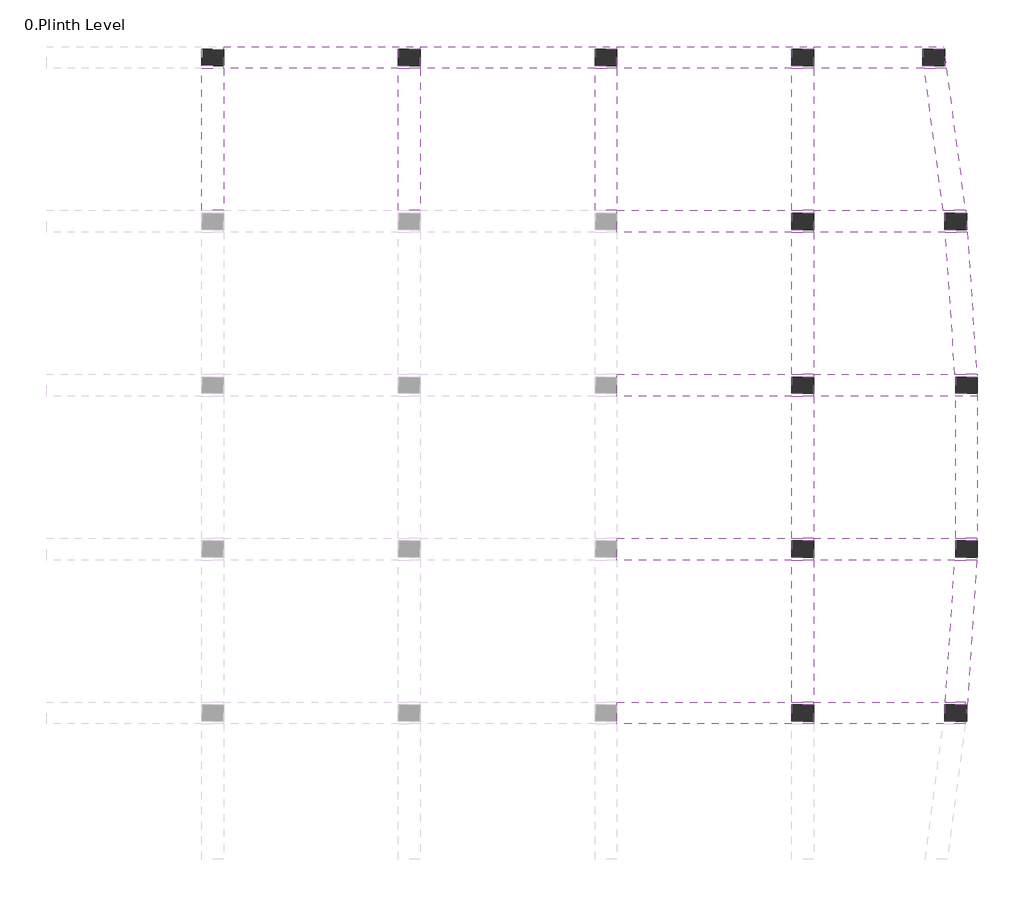
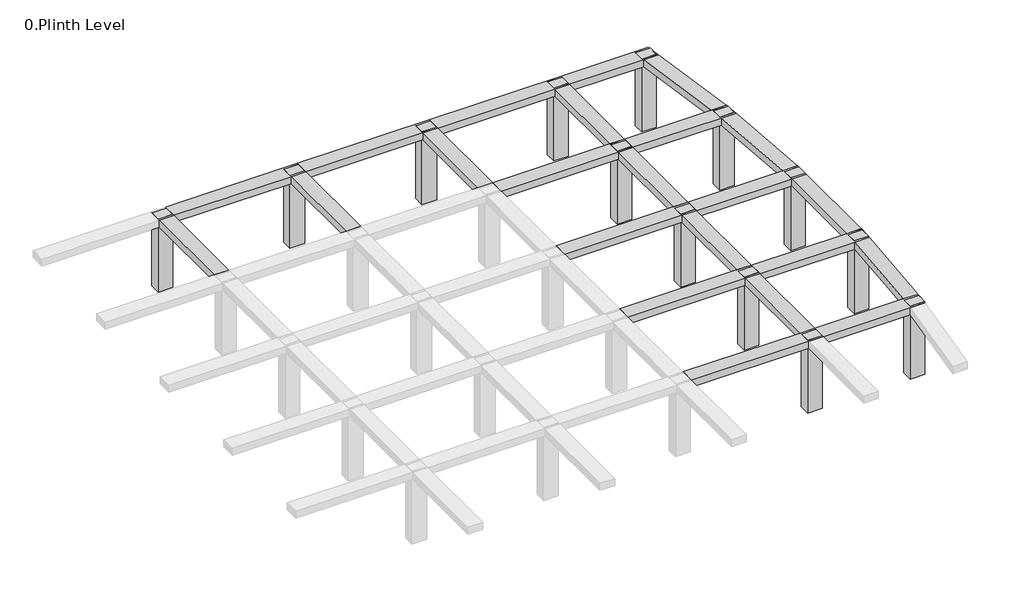
# One storey, part 3 of 3: 23 beams, 13 columns.
"""IFC4 building model written with IfcOpenShell, lengths in millimetres."""

from ifc_helpers import new_model, si_unit, frame, origin, origin_with_axes, place, context, project, spatial, polyline, outline, extrude, faceted_brep, element, save

model = new_model("IFC4")

# Units and contexts
model_context = context("Model", 3, world=origin())
ifc_project = project(units=[si_unit("LENGTHUNIT", "METRE", prefix="MILLI")], contexts=[model_context])

# Site, building, storey
site = spatial("IfcSite", under=ifc_project)
building = spatial("IfcBuilding", under=site)
storey = spatial("IfcBuildingStorey", under=building, Name="0.Plinth Level", Elevation=0.0)

# Beams
placement = place(None, origin())
element("IfcBeam", 1, ObjectType="Concrete-Rectangular Beam : 2' x2'", at=placement, inside=storey, context=model_context, shape_type="Brep", body=[
    faceted_brep([(-160.074232, 1680.7831222, 3200.4), (-160.074232, 1604.5831222, 3200.4), (-160.074232, 1147.3831222, 3200.4), (-160.074232, 1071.1831222, 3200.4), (4716.725768, 1071.1831222, 3200.4), (5326.325768, 1071.1831222, 3200.4), (5326.325768, 1147.3831222, 3200.4), (4716.725768, 1147.3831222, 3200.4), (4716.725768, 1604.5831222, 3200.4), (5326.325768, 1604.5831222, 3200.4), (5326.325768, 1680.7831222, 3200.4), (4716.725768, 1680.7831222, 3200.4), (-160.074232, 1071.1831222, 2895.6), (4716.725768, 1071.1831222, 2895.6), (5326.325768, 1071.1831222, 2895.6), (-160.074232, 1147.3831222, 2895.6), (-160.074232, 1604.5831222, 2895.6), (-160.074232, 1680.7831222, 2895.6), (4716.725768, 1680.7831222, 2895.6), (5326.325768, 1680.7831222, 2895.6), (5326.325768, 1604.5831222, 2895.6), (4716.725768, 1604.5831222, 2895.6), (4716.725768, 1147.3831222, 2895.6), (5326.325768, 1147.3831222, 2895.6)], [[[0, 1, 2, 3, 4, 5, 6, 7, 8, 9, 10, 11]], [[3, 12, 13, 14, 5, 4]], [[12, 15, 16, 17, 18, 19, 20, 21, 22, 23, 14, 13]], [[10, 19, 18, 17, 0, 11]], [[3, 2, 1, 0, 17, 16, 15, 12]], [[5, 14, 23, 6]], [[22, 7, 6, 23]], [[7, 22, 21, 8]], [[8, 21, 20, 9]], [[19, 10, 9, 20]]]),
])
element("IfcBeam", 2, ObjectType="Concrete-Rectangular Beam : 2' x2'", at=placement, inside=storey, context=model_context, shape_type="Brep", body=[
    faceted_brep([(9555.2251658, 1680.7831222, 3200.4), (9003.0522312, 1680.7831222, 3200.4), (5326.325768, 1680.7831222, 3200.4), (5326.325768, 1604.5831222, 3200.4), (5326.325768, 1147.3831222, 3200.4), (5326.325768, 1071.1831222, 3200.4), (8940.2370643, 1071.1831222, 3200.4), (9555.2251658, 1071.1831222, 3200.4), (9555.2251658, 1147.3831222, 3200.4), (8983.5457827, 1147.3831222, 3200.4), (8983.5457827, 1604.5831222, 3200.4), (9555.2251658, 1604.5831222, 3200.4), (9555.2251658, 1071.1831222, 2895.6), (5326.325768, 1071.1831222, 2895.6), (8940.2370643, 1071.1831222, 2895.6), (5326.325768, 1147.3831222, 2895.6), (5326.325768, 1604.5831222, 2895.6), (5326.325768, 1680.7831222, 2895.6), (9003.0522312, 1680.7831222, 2895.6), (9555.2251658, 1680.7831222, 2895.6), (9555.2251658, 1604.5831222, 2895.6), (8983.5457827, 1604.5831222, 2895.6), (8983.5457827, 1147.3831222, 2895.6), (9555.2251658, 1147.3831222, 2895.6)], [[[0, 1, 2, 3, 4, 5, 6, 7, 8, 9, 10, 11]], [[12, 7, 6, 5, 13, 14]], [[12, 14, 13, 15, 16, 17, 18, 19, 20, 21, 22, 23]], [[0, 19, 18, 17, 2, 1]], [[7, 12, 23, 8]], [[5, 4, 3, 2, 17, 16, 15, 13]], [[22, 9, 8, 23]], [[9, 22, 21, 10]], [[10, 21, 20, 11]], [[19, 0, 11, 20]]]),
])
element("IfcBeam", 3, ObjectType="Concrete-Rectangular Beam : 2' x2'", at=placement, inside=storey, context=model_context, shape_type="Brep", body=[
    faceted_brep([(-160.074232, 6252.7831222, 3200.4), (-160.074232, 6176.5831222, 3200.4), (-160.074232, 5719.3831222, 3200.4), (-160.074232, 5643.1831222, 3200.4), (4716.725768, 5643.1831222, 3200.4), (5326.325768, 5643.1831222, 3200.4), (5326.325768, 5719.3831222, 3200.4), (4716.725768, 5719.3831222, 3200.4), (4716.725768, 6176.5831222, 3200.4), (5326.325768, 6176.5831222, 3200.4), (5326.325768, 6252.7831222, 3200.4), (4716.725768, 6252.7831222, 3200.4), (-160.074232, 5643.1831222, 2895.6), (4716.725768, 5643.1831222, 2895.6), (5326.325768, 5643.1831222, 2895.6), (-160.074232, 5719.3831222, 2895.6), (-160.074232, 6176.5831222, 2895.6), (-160.074232, 6252.7831222, 2895.6), (4716.725768, 6252.7831222, 2895.6), (5326.325768, 6252.7831222, 2895.6), (5326.325768, 6176.5831222, 2895.6), (4716.725768, 6176.5831222, 2895.6), (4716.725768, 5719.3831222, 2895.6), (5326.325768, 5719.3831222, 2895.6)], [[[0, 1, 2, 3, 4, 5, 6, 7, 8, 9, 10, 11]], [[3, 12, 13, 14, 5, 4]], [[12, 15, 16, 17, 18, 19, 20, 21, 22, 23, 14, 13]], [[10, 19, 18, 17, 0, 11]], [[3, 2, 1, 0, 17, 16, 15, 12]], [[5, 14, 23, 6]], [[22, 7, 6, 23]], [[7, 22, 21, 8]], [[8, 21, 20, 9]], [[19, 10, 9, 20]]]),
])
element("IfcBeam", 4, ObjectType="Concrete-Rectangular Beam : 2' x2'", at=placement, inside=storey, context=model_context, shape_type="Brep", body=[
    faceted_brep([(9876.2389574, 6252.7831222, 3200.4), (9286.1454059, 6252.7831222, 3200.4), (5326.325768, 6252.7831222, 3200.4), (5326.325768, 6176.5831222, 3200.4), (5326.325768, 5719.3831222, 3200.4), (5326.325768, 5643.1831222, 3200.4), (9265.305238, 5643.1831222, 3200.4), (9876.2389574, 5643.1831222, 3200.4), (9876.2389574, 5719.3831222, 3200.4), (9286.1454059, 5719.3831222, 3200.4), (9286.1454059, 6176.5831222, 3200.4), (9876.2389574, 6176.5831222, 3200.4), (9876.2389574, 5643.1831222, 2895.6), (5326.325768, 5643.1831222, 2895.6), (9265.305238, 5643.1831222, 2895.6), (5326.325768, 5719.3831222, 2895.6), (5326.325768, 6176.5831222, 2895.6), (5326.325768, 6252.7831222, 2895.6), (9286.1454059, 6252.7831222, 2895.6), (9876.2389574, 6252.7831222, 2895.6), (9876.2389574, 6176.5831222, 2895.6), (9286.1454059, 6176.5831222, 2895.6), (9286.1454059, 5719.3831222, 2895.6), (9876.2389574, 5719.3831222, 2895.6)], [[[0, 1, 2, 3, 4, 5, 6, 7, 8, 9, 10, 11]], [[12, 7, 6, 5, 13, 14]], [[12, 14, 13, 15, 16, 17, 18, 19, 20, 21, 22, 23]], [[0, 19, 18, 17, 2, 1]], [[7, 12, 23, 8]], [[5, 4, 3, 2, 17, 16, 15, 13]], [[22, 9, 8, 23]], [[9, 22, 21, 10]], [[10, 21, 20, 11]], [[19, 0, 11, 20]]]),
])
element("IfcBeam", 5, ObjectType="Concrete-Rectangular Beam : 2' x2'", at=placement, inside=storey, context=model_context, shape_type="Brep", body=[
    faceted_brep([(-160.074232, 10824.7831222, 3200.4), (-160.074232, 10748.5831222, 3200.4), (-160.074232, 10291.3831222, 3200.4), (-160.074232, 10215.1831222, 3200.4), (4716.725768, 10215.1831222, 3200.4), (5326.325768, 10215.1831222, 3200.4), (5326.325768, 10291.3831222, 3200.4), (4716.725768, 10291.3831222, 3200.4), (4716.725768, 10748.5831222, 3200.4), (5326.325768, 10748.5831222, 3200.4), (5326.325768, 10824.7831222, 3200.4), (4716.725768, 10824.7831222, 3200.4), (-160.074232, 10215.1831222, 2895.6), (4716.725768, 10215.1831222, 2895.6), (5326.325768, 10215.1831222, 2895.6), (-160.074232, 10291.3831222, 2895.6), (-160.074232, 10748.5831222, 2895.6), (-160.074232, 10824.7831222, 2895.6), (4716.725768, 10824.7831222, 2895.6), (5326.325768, 10824.7831222, 2895.6), (5326.325768, 10748.5831222, 2895.6), (4716.725768, 10748.5831222, 2895.6), (4716.725768, 10291.3831222, 2895.6), (5326.325768, 10291.3831222, 2895.6)], [[[0, 1, 2, 3, 4, 5, 6, 7, 8, 9, 10, 11]], [[3, 12, 13, 14, 5, 4]], [[12, 15, 16, 17, 18, 19, 20, 21, 22, 23, 14, 13]], [[10, 19, 18, 17, 0, 11]], [[3, 2, 1, 0, 17, 16, 15, 12]], [[5, 14, 23, 6]], [[22, 7, 6, 23]], [[7, 22, 21, 8]], [[8, 21, 20, 9]], [[19, 10, 9, 20]]]),
])
element("IfcBeam", 6, ObjectType="Concrete-Rectangular Beam : 2' x2'", at=placement, inside=storey, context=model_context, shape_type="Brep", body=[
    faceted_brep([(9895.7454059, 10824.7831222, 3200.4), (9876.2389574, 10824.7831222, 3200.4), (9265.305238, 10824.7831222, 3200.4), (5326.325768, 10824.7831222, 3200.4), (5326.325768, 10748.5831222, 3200.4), (5326.325768, 10291.3831222, 3200.4), (5326.325768, 10215.1831222, 3200.4), (9895.7454059, 10215.1831222, 3200.4), (9895.7454059, 10291.3831222, 3200.4), (9286.1454059, 10291.3831222, 3200.4), (9286.1454059, 10748.5831222, 3200.4), (9895.7454059, 10748.5831222, 3200.4), (9895.7454059, 10215.1831222, 2895.6), (5326.325768, 10215.1831222, 2895.6), (5326.325768, 10291.3831222, 2895.6), (5326.325768, 10748.5831222, 2895.6), (5326.325768, 10824.7831222, 2895.6), (9265.305238, 10824.7831222, 2895.6), (9876.2389574, 10824.7831222, 2895.6), (9895.7454059, 10824.7831222, 2895.6), (9895.7454059, 10748.5831222, 2895.6), (9286.1454059, 10748.5831222, 2895.6), (9286.1454059, 10291.3831222, 2895.6), (9895.7454059, 10291.3831222, 2895.6)], [[[0, 1, 2, 3, 4, 5, 6, 7, 8, 9, 10, 11]], [[12, 7, 6, 13]], [[12, 13, 14, 15, 16, 17, 18, 19, 20, 21, 22, 23]], [[0, 19, 18, 17, 16, 3, 2, 1]], [[7, 12, 23, 8]], [[6, 5, 4, 3, 16, 15, 14, 13]], [[22, 9, 8, 23]], [[9, 22, 21, 10]], [[10, 21, 20, 11]], [[19, 0, 11, 20]]]),
])
element("IfcBeam", 7, ObjectType="Concrete-Rectangular Beam : 2' x2'", at=placement, inside=storey, context=model_context, shape_type="Brep", body=[
    faceted_brep([(-160.074232, 15396.7831222, 3200.4), (-160.074232, 15320.5831222, 3200.4), (-160.074232, 14863.3831222, 3200.4), (-160.074232, 14787.1831222, 3200.4), (4716.725768, 14787.1831222, 3200.4), (5326.325768, 14787.1831222, 3200.4), (5326.325768, 14863.3831222, 3200.4), (4716.725768, 14863.3831222, 3200.4), (4716.725768, 15320.5831222, 3200.4), (5326.325768, 15320.5831222, 3200.4), (5326.325768, 15396.7831222, 3200.4), (4716.725768, 15396.7831222, 3200.4), (-160.074232, 14787.1831222, 2895.6), (4716.725768, 14787.1831222, 2895.6), (5326.325768, 14787.1831222, 2895.6), (-160.074232, 14863.3831222, 2895.6), (-160.074232, 15320.5831222, 2895.6), (-160.074232, 15396.7831222, 2895.6), (4716.725768, 15396.7831222, 2895.6), (5326.325768, 15396.7831222, 2895.6), (5326.325768, 15320.5831222, 2895.6), (4716.725768, 15320.5831222, 2895.6), (4716.725768, 14863.3831222, 2895.6), (5326.325768, 14863.3831222, 2895.6)], [[[0, 1, 2, 3, 4, 5, 6, 7, 8, 9, 10, 11]], [[3, 12, 13, 14, 5, 4]], [[12, 15, 16, 17, 18, 19, 20, 21, 22, 23, 14, 13]], [[10, 19, 18, 17, 0, 11]], [[3, 2, 1, 0, 17, 16, 15, 12]], [[5, 14, 23, 6]], [[22, 7, 6, 23]], [[7, 22, 21, 8]], [[8, 21, 20, 9]], [[19, 10, 9, 20]]]),
])
element("IfcBeam", 8, ObjectType="Concrete-Rectangular Beam : 2' x2'", at=placement, inside=storey, context=model_context, shape_type="Brep", body=[
    faceted_brep([(9573.6393342, 15396.7831222, 3200.4), (9555.2251658, 15396.7831222, 3200.4), (8940.2370643, 15396.7831222, 3200.4), (5326.325768, 15396.7831222, 3200.4), (5326.325768, 15320.5831222, 3200.4), (5326.325768, 14863.3831222, 3200.4), (5326.325768, 14787.1831222, 3200.4), (9003.0522312, 14787.1831222, 3200.4), (9613.9859506, 14787.1831222, 3200.4), (9593.1457827, 15102.0587543, 3200.4), (9593.1457827, 14863.3831222, 3200.4), (8983.5457827, 14863.3831222, 3200.4), (8983.5457827, 15320.5831222, 3200.4), (9578.6826612, 15320.5831222, 3200.4), (9613.9859506, 14787.1831222, 2895.6), (5326.325768, 14787.1831222, 2895.6), (9003.0522312, 14787.1831222, 2895.6), (5326.325768, 14863.3831222, 2895.6), (5326.325768, 15320.5831222, 2895.6), (5326.325768, 15396.7831222, 2895.6), (8940.2370643, 15396.7831222, 2895.6), (9555.2251658, 15396.7831222, 2895.6), (9573.6393342, 15396.7831222, 2895.6), (9578.6826612, 15320.5831222, 2895.6), (8983.5457827, 15320.5831222, 2895.6), (8983.5457827, 14863.3831222, 2895.6), (9593.1457827, 14863.3831222, 2895.6), (9593.1457827, 15102.0587543, 2895.6)], [[[0, 1, 2, 3, 4, 5, 6, 7, 8, 9, 10, 11, 12, 13]], [[14, 8, 7, 6, 15, 16]], [[14, 16, 15, 17, 18, 19, 20, 21, 22, 23, 24, 25, 26, 27]], [[0, 22, 21, 20, 19, 3, 2, 1]], [[8, 14, 27, 9]], [[6, 5, 4, 3, 19, 18, 17, 15]], [[26, 10, 9, 27]], [[10, 26, 25, 11]], [[11, 25, 24, 12]], [[12, 24, 23, 13]], [[22, 0, 13, 23]]]),
])
element("IfcBeam", 9, ObjectType="Concrete-Rectangular Beam : 2' x2'", at=placement, inside=storey, context=model_context, shape_type="Brep", body=[
    faceted_brep([(-11132.874232, 19968.7831222, 3200.4), (-11132.874232, 19892.5831222, 3200.4), (-11132.874232, 19435.3831222, 3200.4), (-11132.874232, 19359.1831222, 3200.4), (-6256.074232, 19359.1831222, 3200.4), (-5646.474232, 19359.1831222, 3200.4), (-5646.474232, 19435.3831222, 3200.4), (-6256.074232, 19435.3831222, 3200.4), (-6256.074232, 19892.5831222, 3200.4), (-5646.474232, 19892.5831222, 3200.4), (-5646.474232, 19968.7831222, 3200.4), (-11132.874232, 19359.1831222, 2895.6), (-6256.074232, 19359.1831222, 2895.6), (-5646.474232, 19359.1831222, 2895.6), (-11132.874232, 19435.3831222, 2895.6), (-11132.874232, 19892.5831222, 2895.6), (-11132.874232, 19968.7831222, 2895.6), (-5646.474232, 19968.7831222, 2895.6), (-5646.474232, 19892.5831222, 2895.6), (-6256.074232, 19892.5831222, 2895.6), (-6256.074232, 19435.3831222, 2895.6), (-5646.474232, 19435.3831222, 2895.6)], [[[0, 1, 2, 3, 4, 5, 6, 7, 8, 9, 10]], [[3, 11, 12, 13, 5, 4]], [[11, 14, 15, 16, 17, 18, 19, 20, 21, 13, 12]], [[10, 17, 16, 0]], [[3, 2, 1, 0, 16, 15, 14, 11]], [[5, 13, 21, 6]], [[20, 7, 6, 21]], [[7, 20, 19, 8]], [[8, 19, 18, 9]], [[17, 10, 9, 18]]]),
])
element("IfcBeam", 10, ObjectType="Concrete-Rectangular Beam : 2' x2'", at=placement, inside=storey, context=model_context, shape_type="Brep", body=[
    faceted_brep([(-160.074232, 19968.7831222, 3200.4), (-5646.474232, 19968.7831222, 3200.4), (-5646.474232, 19892.5831222, 3200.4), (-5646.474232, 19435.3831222, 3200.4), (-5646.474232, 19359.1831222, 3200.4), (-769.674232, 19359.1831222, 3200.4), (-160.074232, 19359.1831222, 3200.4), (-160.074232, 19435.3831222, 3200.4), (-769.674232, 19435.3831222, 3200.4), (-769.674232, 19892.5831222, 3200.4), (-160.074232, 19892.5831222, 3200.4), (-160.074232, 19359.1831222, 2895.6), (-5646.474232, 19359.1831222, 2895.6), (-769.674232, 19359.1831222, 2895.6), (-5646.474232, 19435.3831222, 2895.6), (-5646.474232, 19892.5831222, 2895.6), (-5646.474232, 19968.7831222, 2895.6), (-160.074232, 19968.7831222, 2895.6), (-160.074232, 19892.5831222, 2895.6), (-769.674232, 19892.5831222, 2895.6), (-769.674232, 19435.3831222, 2895.6), (-160.074232, 19435.3831222, 2895.6)], [[[0, 1, 2, 3, 4, 5, 6, 7, 8, 9, 10]], [[11, 6, 5, 4, 12, 13]], [[11, 13, 12, 14, 15, 16, 17, 18, 19, 20, 21]], [[0, 17, 16, 1]], [[6, 11, 21, 7]], [[4, 3, 2, 1, 16, 15, 14, 12]], [[20, 8, 7, 21]], [[8, 20, 19, 9]], [[9, 19, 18, 10]], [[17, 0, 10, 18]]]),
])
element("IfcBeam", 11, ObjectType="Concrete-Rectangular Beam : 2' x2'", at=placement, inside=storey, context=model_context, shape_type="Brep", body=[
    faceted_brep([(-160.074232, 19968.7831222, 3200.4), (-160.074232, 19892.5831222, 3200.4), (-160.074232, 19435.3831222, 3200.4), (-160.074232, 19359.1831222, 3200.4), (4716.725768, 19359.1831222, 3200.4), (5326.325768, 19359.1831222, 3200.4), (5326.325768, 19435.3831222, 3200.4), (4716.725768, 19435.3831222, 3200.4), (4716.725768, 19892.5831222, 3200.4), (5326.325768, 19892.5831222, 3200.4), (5326.325768, 19968.7831222, 3200.4), (-160.074232, 19359.1831222, 2895.6), (4716.725768, 19359.1831222, 2895.6), (5326.325768, 19359.1831222, 2895.6), (-160.074232, 19435.3831222, 2895.6), (-160.074232, 19892.5831222, 2895.6), (-160.074232, 19968.7831222, 2895.6), (5326.325768, 19968.7831222, 2895.6), (5326.325768, 19892.5831222, 2895.6), (4716.725768, 19892.5831222, 2895.6), (4716.725768, 19435.3831222, 2895.6), (5326.325768, 19435.3831222, 2895.6)], [[[0, 1, 2, 3, 4, 5, 6, 7, 8, 9, 10]], [[3, 11, 12, 13, 5, 4]], [[11, 14, 15, 16, 17, 18, 19, 20, 21, 13, 12]], [[10, 17, 16, 0]], [[3, 2, 1, 0, 16, 15, 14, 11]], [[5, 13, 21, 6]], [[20, 7, 6, 21]], [[7, 20, 19, 8]], [[8, 19, 18, 9]], [[17, 10, 9, 18]]]),
])
element("IfcBeam", 12, ObjectType="Concrete-Rectangular Beam : 2' x2'", at=placement, inside=storey, context=model_context, shape_type="Brep", body=[
    faceted_brep([(5326.325768, 19968.7831222, 3200.4), (5326.325768, 19892.5831222, 3200.4), (5326.325768, 19435.3831222, 3200.4), (5326.325768, 19359.1831222, 3200.4), (8412.2463849, 19359.1831222, 3200.4), (9027.2344863, 19359.1831222, 3200.4), (8983.925768, 19684.2011052, 3200.4), (8983.925768, 19435.3831222, 3200.4), (8374.325768, 19435.3831222, 3200.4), (8374.325768, 19892.5831222, 3200.4), (8956.158818, 19892.5831222, 3200.4), (8946.005151, 19968.7831222, 3200.4), (5326.325768, 19359.1831222, 2895.6), (8412.2463849, 19359.1831222, 2895.6), (9027.2344863, 19359.1831222, 2895.6), (5326.325768, 19435.3831222, 2895.6), (5326.325768, 19892.5831222, 2895.6), (5326.325768, 19968.7831222, 2895.6), (8946.005151, 19968.7831222, 2895.6), (8956.158818, 19892.5831222, 2895.6), (8374.325768, 19892.5831222, 2895.6), (8374.325768, 19435.3831222, 2895.6), (8983.925768, 19435.3831222, 2895.6), (8983.925768, 19684.2011052, 2895.6)], [[[0, 1, 2, 3, 4, 5, 6, 7, 8, 9, 10, 11]], [[3, 12, 13, 14, 5, 4]], [[12, 15, 16, 17, 18, 19, 20, 21, 22, 23, 14, 13]], [[11, 18, 17, 0]], [[3, 2, 1, 0, 17, 16, 15, 12]], [[5, 14, 23, 6]], [[22, 7, 6, 23]], [[7, 22, 21, 8]], [[8, 21, 20, 9]], [[9, 20, 19, 10]], [[18, 11, 10, 19]]]),
])
element("IfcBeam", 13, ObjectType="Concrete-Rectangular Beam : 2' x2'", at=placement, inside=storey, context=model_context, shape_type="SweptSolid", body=[
    extrude(outline(polyline([(-11132.874232, 15396.7831222), (-11742.474232, 15396.7831222), (-11742.474232, 19359.1831222), (-11132.874232, 19359.1831222), (-11132.874232, 15396.7831222)])), frame((0.0, 0.0, 2895.6), z_axis=(0.0, 0.0, 1.0), x_axis=(1.0, 0.0, 0.0)), (0.0, 0.0, 1.0), 304.8),
])
element("IfcBeam", 14, ObjectType="Concrete-Rectangular Beam : 2' x2'", at=placement, inside=storey, context=model_context, shape_type="SweptSolid", body=[
    extrude(outline(polyline([(-5646.474232, 15396.7831222), (-6256.074232, 15396.7831222), (-6256.074232, 19359.1831222), (-5646.474232, 19359.1831222), (-5646.474232, 15396.7831222)])), frame((0.0, 0.0, 2895.6), z_axis=(0.0, 0.0, 1.0), x_axis=(1.0, 0.0, 0.0)), (0.0, 0.0, 1.0), 304.8),
])
element("IfcBeam", 15, ObjectType="Concrete-Rectangular Beam : 2' x2'", at=placement, inside=storey, context=model_context, shape_type="SweptSolid", body=[
    extrude(outline(polyline([(-160.074232, 15396.7831222), (-769.674232, 15396.7831222), (-769.674232, 19359.1831222), (-160.074232, 19359.1831222), (-160.074232, 15396.7831222)])), frame((0.0, 0.0, 2895.6), z_axis=(0.0, 0.0, 1.0), x_axis=(1.0, 0.0, 0.0)), (0.0, 0.0, 1.0), 304.8),
])
element("IfcBeam", 16, ObjectType="Concrete-Rectangular Beam : 2' x2'", at=placement, inside=storey, context=model_context, shape_type="SweptSolid", body=[
    extrude(outline(polyline([(5326.325768, 1680.7831222), (4716.725768, 1680.7831222), (4716.725768, 5643.1831222), (5326.325768, 5643.1831222), (5326.325768, 1680.7831222)])), frame((0.0, 0.0, 2895.6), z_axis=(0.0, 0.0, 1.0), x_axis=(1.0, 0.0, 0.0)), (0.0, 0.0, 1.0), 304.8),
])
element("IfcBeam", 17, ObjectType="Concrete-Rectangular Beam : 2' x2'", at=placement, inside=storey, context=model_context, shape_type="SweptSolid", body=[
    extrude(outline(polyline([(4716.725768, 10215.1831222), (5326.325768, 10215.1831222), (5326.325768, 6252.7831222), (4716.725768, 6252.7831222), (4716.725768, 10215.1831222)])), frame((0.0, 0.0, 2895.6), z_axis=(0.0, 0.0, 1.0), x_axis=(1.0, 0.0, 0.0)), (0.0, 0.0, 1.0), 304.8),
])
element("IfcBeam", 18, ObjectType="Concrete-Rectangular Beam : 2' x2'", at=placement, inside=storey, context=model_context, shape_type="SweptSolid", body=[
    extrude(outline(polyline([(4716.725768, 14787.1831222), (5326.325768, 14787.1831222), (5326.325768, 10824.7831222), (4716.725768, 10824.7831222), (4716.725768, 14787.1831222)])), frame((0.0, 0.0, 2895.6), z_axis=(0.0, 0.0, 1.0), x_axis=(1.0, 0.0, 0.0)), (0.0, 0.0, 1.0), 304.8),
])
element("IfcBeam", 19, ObjectType="Concrete-Rectangular Beam : 2' x2'", at=placement, inside=storey, context=model_context, shape_type="SweptSolid", body=[
    extrude(outline(polyline([(5326.325768, 15396.7831222), (4716.725768, 15396.7831222), (4716.725768, 19359.1831222), (5326.325768, 19359.1831222), (5326.325768, 15396.7831222)])), frame((0.0, 0.0, 2895.6), z_axis=(0.0, 0.0, 1.0), x_axis=(1.0, 0.0, 0.0)), (0.0, 0.0, 1.0), 304.8),
])
element("IfcBeam", 20, ObjectType="Concrete-Rectangular Beam : 2' x2'", at=placement, inside=storey, context=model_context, shape_type="Brep", body=[
    faceted_brep([(9916.5855738, 6252.7831222, 3200.4), (9895.7454059, 6252.7831222, 3200.4), (9876.2389574, 6252.7831222, 3200.4), (9876.2389574, 6176.5831222, 3200.4), (9895.7454059, 6176.5831222, 3200.4), (9895.7454059, 5937.9074901, 3200.4), (9916.5855738, 6252.7831222, 2895.6), (9895.7454059, 5937.9074901, 2895.6), (9876.2389574, 6252.7831222, 2895.6), (9895.7454059, 6252.7831222, 2895.6), (9895.7454059, 6176.5831222, 2895.6), (9876.2389574, 6176.5831222, 2895.6)], [[[0, 1, 2, 3, 4, 5]], [[6, 0, 5, 7]], [[8, 9, 6, 7, 10, 11]], [[0, 6, 9, 8, 2, 1]], [[4, 10, 7, 5]], [[10, 4, 3, 11]], [[2, 8, 11, 3]]]),
    faceted_brep([(9003.0522312, 1680.7831222, 2895.6), (9003.0522312, 1680.7831222, 3200.4), (9265.305238, 5643.1831222, 3200.4), (9265.305238, 5643.1831222, 2895.6), (9021.4663996, 1680.7831222, 2895.6), (9555.2251658, 1680.7831222, 2895.6), (9555.2251658, 1680.7831222, 3200.4), (9021.4663996, 1680.7831222, 3200.4), (9876.2389574, 5643.1831222, 3200.4), (9876.2389574, 5643.1831222, 2895.6), (9876.2389574, 5719.3831222, 3200.4), (9876.2389574, 5719.3831222, 2895.6), (9555.2251658, 1604.5831222, 3200.4), (9593.1457827, 1604.5831222, 3200.4), (9593.1457827, 1365.9074901, 3200.4), (9593.1457827, 1365.9074901, 2895.6), (9593.1457827, 1604.5831222, 2895.6), (9555.2251658, 1604.5831222, 2895.6), (9881.2822845, 5719.3831222, 3200.4), (9881.2822845, 5719.3831222, 2895.6)], [[[0, 1, 2, 3]], [[1, 0, 4, 5, 6, 7]], [[2, 8, 9, 3]], [[9, 8, 10, 11]], [[8, 2, 1, 7, 6, 12, 13, 14]], [[3, 9, 15, 16, 17, 5, 4, 0]], [[13, 16, 15, 14]], [[16, 13, 12, 17]], [[6, 5, 17, 12]], [[10, 18, 19, 11]], [[10, 8, 18]], [[8, 14, 15, 9, 19, 18]], [[19, 9, 11]]]),
    faceted_brep([(9555.2251658, 1071.1831222, 3200.4), (9555.2251658, 1071.1831222, 2895.6), (9565.3788327, 1147.3831222, 2895.6), (9565.3788327, 1147.3831222, 3200.4), (9555.2251658, 1147.3831222, 3200.4), (9555.2251658, 1147.3831222, 2895.6)], [[[0, 1, 2, 3]], [[1, 0, 4, 5]], [[3, 2, 5, 4]], [[4, 0, 3]], [[2, 1, 5]]]),
])
element("IfcBeam", 21, ObjectType="Concrete-Rectangular Beam : 2' x2'", at=placement, inside=storey, context=model_context, shape_type="Brep", body=[
    faceted_brep([(9895.7454059, 10824.7831222, 3200.4), (9876.2389574, 10824.7831222, 3200.4), (9286.1454059, 10824.7831222, 3200.4), (9286.1454059, 10748.5831222, 3200.4), (9895.7454059, 10748.5831222, 3200.4), (9895.7454059, 10824.7831222, 2895.6), (9895.7454059, 10748.5831222, 2895.6), (9286.1454059, 10824.7831222, 2895.6), (9876.2389574, 10824.7831222, 2895.6), (9286.1454059, 10748.5831222, 2895.6)], [[[0, 1, 2, 3, 4]], [[5, 0, 4, 6]], [[7, 8, 5, 6, 9]], [[2, 7, 9, 3]], [[2, 1, 0, 5, 8, 7]], [[4, 3, 9, 6]]]),
    faceted_brep([(9286.1454059, 6252.7831222, 3200.4), (9286.1454059, 6252.7831222, 2895.6), (9876.2389574, 6252.7831222, 2895.6), (9895.7454059, 6252.7831222, 2895.6), (9895.7454059, 6252.7831222, 3200.4), (9876.2389574, 6252.7831222, 3200.4), (9286.1454059, 10291.3831222, 3200.4), (9895.7454059, 10291.3831222, 3200.4), (9895.7454059, 10291.3831222, 2895.6), (9286.1454059, 10291.3831222, 2895.6)], [[[0, 1, 2, 3, 4, 5]], [[6, 7, 8, 9]], [[0, 5, 4, 7, 6]], [[4, 3, 8, 7]], [[3, 2, 1, 9, 8]], [[1, 0, 6, 9]]]),
])
element("IfcBeam", 22, ObjectType="Concrete-Rectangular Beam : 2' x2'", at=placement, inside=storey, context=model_context, shape_type="Brep", body=[
    faceted_brep([(9613.9859506, 14787.1831222, 3200.4), (9003.0522312, 14787.1831222, 3200.4), (9265.305238, 10824.7831222, 3200.4), (9286.1454059, 10824.7831222, 3200.4), (9876.2389574, 10824.7831222, 3200.4), (9613.9859506, 14787.1831222, 2895.6), (9876.2389574, 10824.7831222, 2895.6), (9003.0522312, 14787.1831222, 2895.6), (9286.1454059, 10824.7831222, 2895.6), (9265.305238, 10824.7831222, 2895.6)], [[[0, 1, 2, 3, 4]], [[5, 0, 4, 6]], [[7, 5, 6, 8, 9]], [[1, 7, 9, 2]], [[1, 0, 5, 7]], [[4, 3, 2, 9, 8, 6]]]),
])
element("IfcBeam", 23, ObjectType="Concrete-Rectangular Beam : 2' x2'", at=placement, inside=storey, context=model_context, shape_type="SweptSolid", body=[
    extrude(outline(polyline([(8412.2463849, 19359.1831222), (9027.2344863, 19359.1831222), (9555.2251658, 15396.7831222), (8940.2370643, 15396.7831222), (8412.2463849, 19359.1831222)])), frame((0.0, 0.0, 2895.6), z_axis=(0.0, 0.0, 1.0), x_axis=(1.0, 0.0, 0.0)), (0.0, 0.0, 1.0), 304.8),
])

# Columns
element("IfcColumn", 24, ObjectType="Concrete-Rectangular-Column : 12 x 18", at=placement, inside=storey, context=model_context, shape_type="SweptSolid", body=[
    extrude(outline(polyline([(5326.325768, 1604.5831222), (5326.325768, 1147.3831222), (4716.725768, 1147.3831222), (4716.725768, 1604.5831222), (5326.325768, 1604.5831222)])), origin_with_axes(), (0.0, 0.0, 1.0), 3200.4),
])
element("IfcColumn", 25, ObjectType="Concrete-Rectangular-Column : 12 x 18", at=placement, inside=storey, context=model_context, shape_type="SweptSolid", body=[
    extrude(outline(polyline([(9593.1457827, 1604.5831222), (9593.1457827, 1147.3831222), (8983.5457827, 1147.3831222), (8983.5457827, 1604.5831222), (9593.1457827, 1604.5831222)])), origin_with_axes(), (0.0, 0.0, 1.0), 3200.4),
])
element("IfcColumn", 26, ObjectType="Concrete-Rectangular-Column : 12 x 18", at=placement, inside=storey, context=model_context, shape_type="SweptSolid", body=[
    extrude(outline(polyline([(5326.325768, 6176.5831222), (5326.325768, 5719.3831222), (4716.725768, 5719.3831222), (4716.725768, 6176.5831222), (5326.325768, 6176.5831222)])), origin_with_axes(), (0.0, 0.0, 1.0), 3200.4),
])
element("IfcColumn", 27, ObjectType="Concrete-Rectangular-Column : 12 x 18", at=placement, inside=storey, context=model_context, shape_type="SweptSolid", body=[
    extrude(outline(polyline([(9895.7454059, 6176.5831222), (9895.7454059, 5719.3831222), (9286.1454059, 5719.3831222), (9286.1454059, 6176.5831222), (9895.7454059, 6176.5831222)])), origin_with_axes(), (0.0, 0.0, 1.0), 3200.4),
])
element("IfcColumn", 28, ObjectType="Concrete-Rectangular-Column : 12 x 18", at=placement, inside=storey, context=model_context, shape_type="SweptSolid", body=[
    extrude(outline(polyline([(5326.325768, 10748.5831222), (5326.325768, 10291.3831222), (4716.725768, 10291.3831222), (4716.725768, 10748.5831222), (5326.325768, 10748.5831222)])), origin_with_axes(), (0.0, 0.0, 1.0), 3200.4),
])
element("IfcColumn", 29, ObjectType="Concrete-Rectangular-Column : 12 x 18", at=placement, inside=storey, context=model_context, shape_type="SweptSolid", body=[
    extrude(outline(polyline([(9895.7454059, 10748.5831222), (9895.7454059, 10291.3831222), (9286.1454059, 10291.3831222), (9286.1454059, 10748.5831222), (9895.7454059, 10748.5831222)])), origin_with_axes(), (0.0, 0.0, 1.0), 3200.4),
])
element("IfcColumn", 30, ObjectType="Concrete-Rectangular-Column : 12 x 18", at=placement, inside=storey, context=model_context, shape_type="SweptSolid", body=[
    extrude(outline(polyline([(5326.325768, 15320.5831222), (5326.325768, 14863.3831222), (4716.725768, 14863.3831222), (4716.725768, 15320.5831222), (5326.325768, 15320.5831222)])), origin_with_axes(), (0.0, 0.0, 1.0), 3200.4),
])
element("IfcColumn", 31, ObjectType="Concrete-Rectangular-Column : 12 x 18", at=placement, inside=storey, context=model_context, shape_type="SweptSolid", body=[
    extrude(outline(polyline([(9593.1457827, 15320.5831222), (9593.1457827, 14863.3831222), (8983.5457827, 14863.3831222), (8983.5457827, 15320.5831222), (9593.1457827, 15320.5831222)])), origin_with_axes(), (0.0, 0.0, 1.0), 3200.4),
])
element("IfcColumn", 32, ObjectType="Concrete-Rectangular-Column : 12 x 18", at=placement, inside=storey, context=model_context, shape_type="SweptSolid", body=[
    extrude(outline(polyline([(-11132.874232, 19892.5831222), (-11132.874232, 19435.3831222), (-11742.474232, 19435.3831222), (-11742.474232, 19892.5831222), (-11132.874232, 19892.5831222)])), origin_with_axes(), (0.0, 0.0, 1.0), 3200.4),
])
element("IfcColumn", 33, ObjectType="Concrete-Rectangular-Column : 12 x 18", at=placement, inside=storey, context=model_context, shape_type="SweptSolid", body=[
    extrude(outline(polyline([(-5646.474232, 19892.5831222), (-5646.474232, 19435.3831222), (-6256.074232, 19435.3831222), (-6256.074232, 19892.5831222), (-5646.474232, 19892.5831222)])), origin_with_axes(), (0.0, 0.0, 1.0), 3200.4),
])
element("IfcColumn", 34, ObjectType="Concrete-Rectangular-Column : 12 x 18", at=placement, inside=storey, context=model_context, shape_type="SweptSolid", body=[
    extrude(outline(polyline([(-160.074232, 19892.5831222), (-160.074232, 19435.3831222), (-769.674232, 19435.3831222), (-769.674232, 19892.5831222), (-160.074232, 19892.5831222)])), origin_with_axes(), (0.0, 0.0, 1.0), 3200.4),
])
element("IfcColumn", 35, ObjectType="Concrete-Rectangular-Column : 12 x 18", at=placement, inside=storey, context=model_context, shape_type="SweptSolid", body=[
    extrude(outline(polyline([(5326.325768, 19892.5831222), (5326.325768, 19435.3831222), (4716.725768, 19435.3831222), (4716.725768, 19892.5831222), (5326.325768, 19892.5831222)])), origin_with_axes(), (0.0, 0.0, 1.0), 3200.4),
])
element("IfcColumn", 36, ObjectType="Concrete-Rectangular-Column : 12 x 18", at=placement, inside=storey, context=model_context, shape_type="SweptSolid", body=[
    extrude(outline(polyline([(8983.925768, 19892.5831222), (8983.925768, 19435.3831222), (8374.325768, 19435.3831222), (8374.325768, 19892.5831222), (8983.925768, 19892.5831222)])), origin_with_axes(), (0.0, 0.0, 1.0), 3200.4),
])

save(model, "model.ifc")

# Revit data of these elements
# Type "Concrete-Rectangular Beam : 2' x2'"
#   Assembly Code = "B10"
#   Length [instance default] = 5' - 0"
#   b = 2' - 0"
#   h = 1' - 0"
#   Structural Material [instance default] = Concrete, Cast-in-Place gray
# Type "Concrete-Rectangular-Column : 12 x 18"
#   Assembly Code = "B10"
#   b = 2' - 0"
#   h = 1' - 6"
#   Structural Material [instance default] = Concrete, Cast-in-Place gray
# Elements 1, 2, 3, 4, 5, 6, 7, 8, 9, 10, 11, 12, 13, 14, 15, 16, 17, 18, 19, 20, 21, 22, 23 (IfcBeam, "Concrete-Rectangular Beam : 2' x2'")
#   Structural Material = Concrete, Precast (2)
#   Phase Created = New Construction
#   Materials on its faces: "Concrete, Precast (2)"
# Elements 24, 25, 26, 27, 28, 29, 30, 31, 32, 33, 34, 35, 36 (IfcColumn, "Concrete-Rectangular-Column : 12 x 18")
#   Phase Created = New Construction
#   Materials on its faces: "Concrete, Cast-in-Place gray"
# Materials
#   "Concrete, Cast-in-Place gray": class "Concrete", colour RGB 192 192 192, transparency 0, Description = "Cast-in-place concrete", Cost = 0
#   "Concrete, Precast (2)": class "Concrete", colour RGB 198 187 187, transparency 0, Description = "Precast concrete", Cost = 0
